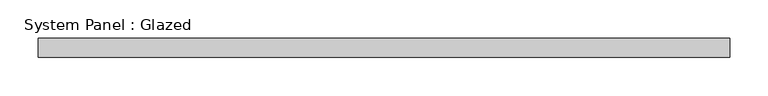
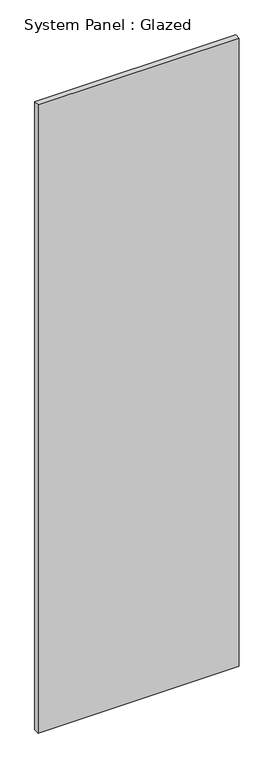
"""IFC4 building model written with IfcOpenShell, lengths in millimetres: plate geometry, System Panel : Glazed."""

from ifc_helpers import new_model, si_unit, origin, origin_with_axes, place, context, project, spatial, polyline, outline, extrude, source, transform, mapped, element, save


def system_panel_glazed_8fd4c810(model_context):
    return source(origin(), model_context, "Body", "SweptSolid", [
        extrude(outline(polyline([(454.025, 24.5), (-454.025, 24.5), (-454.025, 49.5), (454.025, 49.5), (454.025, 24.5)])), origin_with_axes(), (0.0, 0.0, 1.0), 3000.0),
    ])


if __name__ == "__main__":
    model = new_model("IFC4")
    model_context = context("Model", 3, world=origin())
    ifc_project = project(units=[si_unit("LENGTHUNIT", "METRE", prefix="MILLI")], contexts=[model_context])
    site = spatial("IfcSite", under=ifc_project)
    building = spatial("IfcBuilding", under=site)
    placement = place(None, origin())
    system_panel_glazed_shape = system_panel_glazed_8fd4c810(model_context)
    element("IfcPlate", 1, ObjectType="System Panel : Glazed", at=placement, inside=building, context=model_context, shape_type="MappedRepresentation", body=[
        mapped(system_panel_glazed_shape, transform((0.0, 0.0, 0.0), x_axis=(1.0, 0.0, 0.0), y_axis=(0.0, 1.0, 0.0), z_axis=(0.0, 0.0, 1.0))),
    ])
    save(model, "model.ifc")

# Revit data of these elements
# Type "System Panel : Glazed"
#   Keynote = "H11"
#   Construction Type Id = "GSP4R"
#   Analytic Construction = "1/8 in Pilkington single glazing"
#   Visual Light Transmittance = 0.9
#   Solar Heat Gain Coefficient = 0.86
#   Heat Transfer Coefficient (U) = 6.7069 W/(m²·K)
#   Define Thermal Properties by = 1
# Element 1 (IfcPlate, "System Panel : Glazed")
#   Materials on its faces: "Glass"
# Materials
#   "Glass": class "Glass", colour RGB 0 128 192, transparency 0.9, Description = "Soda Lime Glass", Cost = 0
